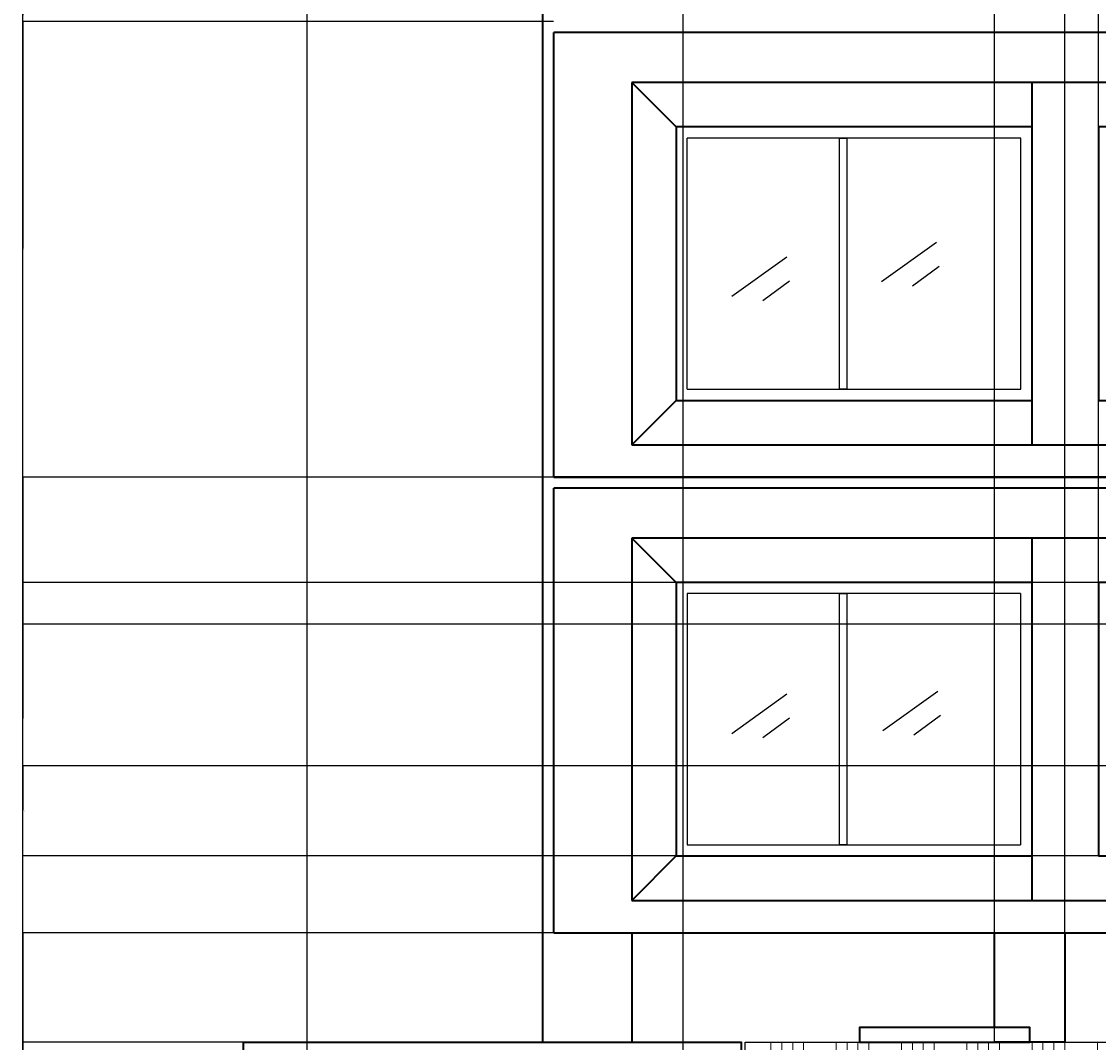
# Model space of a CAD drawing. Units: inches. Extents: x -97 to 1206, y -378 to 680.
# Tile 2 of 6: x -97 to 194, y -25 to 251. Entities that reach past the tile are written whole.
import ezdxf

# ---------------------------------------------------------------- set-up
doc = ezdxf.new("R2010")
doc.units = ezdxf.units.IN
doc.header["$MEASUREMENT"] = 0
for name, color, linetype, lineweight in [('A-ANNO-DIMS', 2, 'Continuous', 18), ('A-DOOR', 3, 'Continuous', 25), ('A-ELEV', 7, 'Continuous', 35), ('A-ELEV-PATT', 252, 'Continuous', 13), ('A-GLAZ', 4, 'Continuous', 25)]:
    doc.layers.add(name, color=color, linetype=linetype, lineweight=lineweight)
doc.styles.get("Standard").update_dxf_attribs({"font": 'arial.ttf'})
doc.dimstyles.get("Standard").update_dxf_attribs({"dimtxt": 0.18, "dimasz": 0.18, "dimexe": 0.18, "dimexo": 0.0625, "dimgap": 0.09, "dimtad": 0, "dimtih": 1, "dimtoh": 1, "dimdec": 4, "dimzin": 0, "dimdsep": 46, "dimtxsty": 'Standard', "dimcen": 0.09, "dimadec": 0, "dimazin": 0, "dimtfac": 1, "dimtdec": 4, "dimtofl": 0, "dimtmove": 0, "dimatfit": 3, "dimfxl": 1, "dimtolj": 1, "dimtzin": 0, "dimarcsym": 0})

# ---------------------------------------------------------------- blocks, each defined once
blk = doc.blocks.new('FACADE-SURROUND')
for p, q in [((432, 97.83), (0, 97.83)), ((0, 97.83), (0, 0)), ((12, 85.83), (0, 97.83)), ((300, 85.83), (312, 97.83)), ((312, 0), (312, 97.83)), ((312, 0), (312, 97.83)), ((312, 97.83), (324, 85.83)), ((432, 97.83), (420, 85.83)), ((432, 0), (432, 97.83)), ((12, 85.83), (12, 12)), ((108, 85.83), (12, 85.83)), ((300, 85.83), (126, 85.83)), ((126, 85.83), (126, 12)), ((300, 12), (300, 85.83)), ((324, 12), (324, 85.83)), ((420, 85.83), (324, 85.83)), ((420, 12), (420, 85.83)), ((12, 12), (0, 0)), ((12, 12), (108, 12)), ((126, 12), (300, 12)), ((300, 12), (312, 0)), ((312, 0), (324, 12)), ((324, 12), (420, 12)), ((432, 0), (420, 12)), ((0, 0), (432, 0))]:
    blk.add_line(p, q)
blk = doc.blocks.new('WIN-1500')
for p, q in [((90, 67.83), (0, 67.83)), ((0, 67.83), (0, 0)), ((90, 67.83), (90, 0)), ((0, 0), (90, 0))]:
    blk.add_line(p, q)
blk = doc.blocks.new('*D12')
at = {"layer": 'A-ANNO-DIMS', "color": 0, "lineweight": -2, "transparency": 16777216}
for p, q in [((43.86, 619.86), (-96.59, 619.86)), ((-96.41, 619.68), (-96.41, 252.54)), ((-96.41, -114.96), (-96.41, 252.17)), ((-36.97, -115.14), (-96.59, -115.14))]:
    blk.add_line(p, q, dxfattribs=at)
at = {"layer": 'A-ANNO-DIMS', "color": 0, "transparency": 16777216}
for points in [[(-96.44, 619.68), (-96.38, 619.68), (-96.41, 619.86)], [(-96.44, -114.96), (-96.38, -114.96), (-96.41, -115.14)]]:
    blk.add_solid(points, dxfattribs=at)
at = {"layer": 'Defpoints', "color": 0, "transparency": 16777216}
for p in [(43.93, 619.86), (-96.41, -115.14), (-36.91, -115.14)]:
    blk.add_point(p, dxfattribs=at)
at = {"layer": 'A-ANNO-DIMS', "color": 0, "transparency": 16777216, "insert": (-96.41, 252.36), "char_height": 0.18, "attachment_point": 5}
blk.add_mtext('\\A1;735', dxfattribs=at)
blk = doc.blocks.new('*D13')
at = {"layer": 'A-ANNO-DIMS', "color": 0, "lineweight": -2, "transparency": 16777216}
for p, q in [((46.86, 4.86), (-96.59, 4.86)), ((-96.41, 4.68), (-96.41, -54.96)), ((-96.41, -114.96), (-96.41, -55.33)), ((-36.97, -115.14), (-96.59, -115.14))]:
    blk.add_line(p, q, dxfattribs=at)
at = {"layer": 'A-ANNO-DIMS', "color": 0, "transparency": 16777216}
for points in [[(-96.44, 4.68), (-96.38, 4.68), (-96.41, 4.86)], [(-96.44, -114.96), (-96.38, -114.96), (-96.41, -115.14)]]:
    blk.add_solid(points, dxfattribs=at)
at = {"layer": 'Defpoints', "color": 0, "transparency": 16777216}
for p in [(46.93, 4.86), (-96.41, -115.14), (-36.91, -115.14)]:
    blk.add_point(p, dxfattribs=at)
at = {"layer": 'A-ANNO-DIMS', "color": 0, "transparency": 16777216, "insert": (-96.41, -55.14), "char_height": 0.18, "attachment_point": 5}
blk.add_mtext('\\A1;120', dxfattribs=at)
blk = doc.blocks.new('*D14')
at = {"layer": 'A-ANNO-DIMS', "color": 0, "lineweight": -2, "transparency": 16777216}
for p, q in [((46.86, 127.86), (-96.59, 127.86)), ((-96.41, 127.68), (-96.41, 66.54)), ((-96.41, 5.04), (-96.41, 66.17)), ((46.86, 4.86), (-96.59, 4.86))]:
    blk.add_line(p, q, dxfattribs=at)
at = {"layer": 'A-ANNO-DIMS', "color": 0, "transparency": 16777216}
for points in [[(-96.44, 127.68), (-96.38, 127.68), (-96.41, 127.86)], [(-96.44, 5.04), (-96.38, 5.04), (-96.41, 4.86)]]:
    blk.add_solid(points, dxfattribs=at)
at = {"layer": 'Defpoints', "color": 0, "transparency": 16777216}
for p in [(-96.41, 127.86), (46.93, 127.86), (46.93, 4.86)]:
    blk.add_point(p, dxfattribs=at)
at = {"layer": 'A-ANNO-DIMS', "color": 0, "transparency": 16777216, "insert": (-96.41, 66.36), "char_height": 0.18, "attachment_point": 5}
blk.add_mtext('\\A1;123', dxfattribs=at)
blk = doc.blocks.new('*D15')
at = {"layer": 'A-ANNO-DIMS', "color": 0, "lineweight": -2, "transparency": 16777216}
for p, q in [((46.86, 250.86), (-96.59, 250.86)), ((-96.41, 250.68), (-96.41, 189.54)), ((-96.41, 128.04), (-96.41, 189.17)), ((46.86, 127.86), (-96.59, 127.86))]:
    blk.add_line(p, q, dxfattribs=at)
at = {"layer": 'A-ANNO-DIMS', "color": 0, "transparency": 16777216}
for points in [[(-96.44, 250.68), (-96.38, 250.68), (-96.41, 250.86)], [(-96.44, 128.04), (-96.38, 128.04), (-96.41, 127.86)]]:
    blk.add_solid(points, dxfattribs=at)
at = {"layer": 'Defpoints', "color": 0, "transparency": 16777216}
for p in [(-96.41, 250.86), (46.93, 250.86), (46.93, 127.86)]:
    blk.add_point(p, dxfattribs=at)
at = {"layer": 'A-ANNO-DIMS', "color": 0, "transparency": 16777216, "insert": (-96.41, 189.36), "char_height": 0.18, "attachment_point": 5}
blk.add_mtext('\\A1;123', dxfattribs=at)
blk = doc.blocks.new('*D16')
at = {"layer": 'A-ANNO-DIMS', "color": 0, "lineweight": -2, "transparency": 16777216}
for p, q in [((46.86, 373.86), (-96.59, 373.86)), ((-96.41, 373.68), (-96.41, 312.54)), ((-96.41, 251.04), (-96.41, 312.17)), ((46.86, 250.86), (-96.59, 250.86))]:
    blk.add_line(p, q, dxfattribs=at)
at = {"layer": 'A-ANNO-DIMS', "color": 0, "transparency": 16777216}
for points in [[(-96.44, 373.68), (-96.38, 373.68), (-96.41, 373.86)], [(-96.44, 251.04), (-96.38, 251.04), (-96.41, 250.86)]]:
    blk.add_solid(points, dxfattribs=at)
at = {"layer": 'Defpoints', "color": 0, "transparency": 16777216}
for p in [(-96.41, 373.86), (46.93, 373.86), (46.93, 250.86)]:
    blk.add_point(p, dxfattribs=at)
at = {"layer": 'A-ANNO-DIMS', "color": 0, "transparency": 16777216, "insert": (-96.41, 312.36), "char_height": 0.18, "attachment_point": 5}
blk.add_mtext('\\A1;123', dxfattribs=at)
blk = doc.blocks.new('*D35')
at = {"layer": 'A-ANNO-DIMS', "color": 0, "lineweight": -2, "transparency": 16777216}
for p, q in [((-36.97, -24.73), (-96.59, -24.73)), ((-96.41, -24.91), (-96.41, -69.75)), ((-96.41, -114.96), (-96.41, -70.12)), ((-36.97, -115.14), (-96.59, -115.14))]:
    blk.add_line(p, q, dxfattribs=at)
at = {"layer": 'A-ANNO-DIMS', "color": 0, "transparency": 16777216}
for points in [[(-96.44, -24.91), (-96.38, -24.91), (-96.41, -24.73)], [(-96.44, -114.96), (-96.38, -114.96), (-96.41, -115.14)]]:
    blk.add_solid(points, dxfattribs=at)
at = {"layer": 'Defpoints', "color": 0, "transparency": 16777216}
for p in [(-96.41, -24.73), (-36.91, -24.73), (-36.91, -115.14)]:
    blk.add_point(p, dxfattribs=at)
at = {"layer": 'A-ANNO-DIMS', "color": 0, "transparency": 16777216, "insert": (-96.41, -69.94), "char_height": 0.18, "attachment_point": 5}
blk.add_mtext('\\A1;90.42', dxfattribs=at)
blk = doc.blocks.new('*D36')
at = {"layer": 'A-ANNO-DIMS', "color": 0, "lineweight": -2, "transparency": 16777216}
for p, q in [((-19.68, -48.26), (-19.68, 679.54)), ((-19.5, 679.36), (30.69, 679.36)), ((81.65, 679.36), (31.46, 679.36)), ((81.83, -48.26), (81.83, 679.54))]:
    blk.add_line(p, q, dxfattribs=at)
at = {"layer": 'A-ANNO-DIMS', "color": 0, "transparency": 16777216}
for points in [[(-19.5, 679.39), (-19.5, 679.33), (-19.68, 679.36)], [(81.65, 679.39), (81.65, 679.33), (81.83, 679.36)]]:
    blk.add_solid(points, dxfattribs=at)
at = {"layer": 'Defpoints', "color": 0, "transparency": 16777216}
for p in [(81.83, 679.36), (-19.68, -48.33), (81.83, -48.33)]:
    blk.add_point(p, dxfattribs=at)
at = {"layer": 'A-ANNO-DIMS', "color": 0, "transparency": 16777216, "insert": (31.08, 679.36), "char_height": 0.18, "attachment_point": 5}
blk.add_mtext('\\A1;101.5', dxfattribs=at)
blk = doc.blocks.new('*D40')
at = {"layer": 'A-ANNO-DIMS', "color": 0, "lineweight": -2, "transparency": 16777216}
for p, q in [((193.93, 99.46), (193.93, 679.54)), ((194.11, 679.36), (280.65, 679.36)), ((367.75, 679.36), (281.21, 679.36)), ((367.93, 99.46), (367.93, 679.54))]:
    blk.add_line(p, q, dxfattribs=at)
at = {"layer": 'A-ANNO-DIMS', "color": 0, "transparency": 16777216}
for points in [[(194.11, 679.39), (194.11, 679.33), (193.93, 679.36)], [(367.75, 679.39), (367.75, 679.33), (367.93, 679.36)]]:
    blk.add_solid(points, dxfattribs=at)
at = {"layer": 'Defpoints', "color": 0, "transparency": 16777216}
for p in [(367.93, 679.36), (193.93, 99.4), (367.93, 99.4)]:
    blk.add_point(p, dxfattribs=at)
at = {"layer": 'A-ANNO-DIMS', "color": 0, "transparency": 16777216, "insert": (280.93, 679.36), "char_height": 0.18, "attachment_point": 5}
blk.add_mtext('\\A1;174', dxfattribs=at)
blk = doc.blocks.new('*D41')
at = {"layer": 'A-ANNO-DIMS', "color": 0, "lineweight": -2, "transparency": 16777216}
for p, q in [((193.86, 99.4), (-96.59, 99.4)), ((-96.41, 99.22), (-96.41, 62.66)), ((-96.41, 25.75), (-96.41, 62.3)), ((193.86, 25.57), (-96.59, 25.57))]:
    blk.add_line(p, q, dxfattribs=at)
at = {"layer": 'A-ANNO-DIMS', "color": 0, "transparency": 16777216}
for points in [[(-96.44, 99.22), (-96.38, 99.22), (-96.41, 99.4)], [(-96.44, 25.75), (-96.38, 25.75), (-96.41, 25.57)]]:
    blk.add_solid(points, dxfattribs=at)
at = {"layer": 'Defpoints', "color": 0, "transparency": 16777216}
for p in [(-96.41, 99.4), (193.93, 99.4), (193.93, 25.57)]:
    blk.add_point(p, dxfattribs=at)
at = {"layer": 'A-ANNO-DIMS', "color": 0, "transparency": 16777216, "insert": (-96.41, 62.48), "char_height": 0.18, "attachment_point": 5}
blk.add_mtext('\\A1;73.83', dxfattribs=at)
blk = doc.blocks.new('*D42')
at = {"layer": 'A-ANNO-DIMS', "color": 0, "lineweight": -2, "transparency": 16777216}
for p, q in [((193.86, 49.88), (-96.59, 49.88)), ((-96.41, 49.7), (-96.41, 37.91)), ((-96.41, 25.75), (-96.41, 37.54)), ((193.86, 25.57), (-96.59, 25.57))]:
    blk.add_line(p, q, dxfattribs=at)
at = {"layer": 'A-ANNO-DIMS', "color": 0, "transparency": 16777216}
for points in [[(-96.44, 49.7), (-96.38, 49.7), (-96.41, 49.88)], [(-96.44, 25.75), (-96.38, 25.75), (-96.41, 25.57)]]:
    blk.add_solid(points, dxfattribs=at)
at = {"layer": 'Defpoints', "color": 0, "transparency": 16777216}
for p in [(-96.41, 49.88), (193.93, 49.88), (193.93, 25.57)]:
    blk.add_point(p, dxfattribs=at)
at = {"layer": 'A-ANNO-DIMS', "color": 0, "transparency": 16777216, "insert": (-96.41, 37.72), "char_height": 0.18, "attachment_point": 5}
blk.add_mtext('\\A1;24.314', dxfattribs=at)
blk = doc.blocks.new('*D44')
at = {"layer": 'A-ANNO-DIMS', "color": 0, "lineweight": -2, "transparency": 16777216}
for p, q in [((262.43, 88.15), (-96.59, 88.15)), ((-96.41, 87.97), (-96.41, 69.2)), ((-96.41, 50.06), (-96.41, 68.83)), ((262.43, 49.88), (-96.59, 49.88))]:
    blk.add_line(p, q, dxfattribs=at)
at = {"layer": 'A-ANNO-DIMS', "color": 0, "transparency": 16777216}
for points in [[(-96.44, 87.97), (-96.38, 87.97), (-96.41, 88.15)], [(-96.44, 50.06), (-96.38, 50.06), (-96.41, 49.88)]]:
    blk.add_solid(points, dxfattribs=at)
at = {"layer": 'Defpoints', "color": 0, "transparency": 16777216}
for p in [(-96.41, 88.15), (262.49, 88.15), (262.49, 49.88)]:
    blk.add_point(p, dxfattribs=at)
at = {"layer": 'A-ANNO-DIMS', "color": 0, "transparency": 16777216, "insert": (-96.41, 69.01), "char_height": 0.18, "attachment_point": 5}
blk.add_mtext('\\A1;38.266', dxfattribs=at)
blk = doc.blocks.new('*D45')
at = {"layer": 'A-ANNO-DIMS', "color": 0, "lineweight": -2, "transparency": 16777216}
for p, q in [((43.93, -24.66), (43.93, 679.54)), ((44.11, 679.36), (104.5, 679.36)), ((165.65, 679.36), (105.27, 679.36)), ((165.83, -24.66), (165.83, 679.54))]:
    blk.add_line(p, q, dxfattribs=at)
at = {"layer": 'A-ANNO-DIMS', "color": 0, "transparency": 16777216}
for points in [[(44.11, 679.39), (44.11, 679.33), (43.93, 679.36)], [(165.65, 679.39), (165.65, 679.33), (165.83, 679.36)]]:
    blk.add_solid(points, dxfattribs=at)
at = {"layer": 'Defpoints', "color": 0, "transparency": 16777216}
for p in [(165.83, 679.36), (43.93, -24.73), (165.83, -24.73)]:
    blk.add_point(p, dxfattribs=at)
at = {"layer": 'A-ANNO-DIMS', "color": 0, "transparency": 16777216, "insert": (104.88, 679.36), "char_height": 0.18, "attachment_point": 5}
blk.add_mtext('\\A1;121.9', dxfattribs=at)
blk = doc.blocks.new('*D46')
at = {"layer": 'A-ANNO-DIMS', "color": 0, "lineweight": -2, "transparency": 16777216}
for p, q in [((165.83, -24.66), (165.83, 679.54)), ((166.01, 679.36), (174.88, 679.36)), ((184.65, 679.36), (175.79, 679.36)), ((184.83, -24.66), (184.83, 679.54))]:
    blk.add_line(p, q, dxfattribs=at)
at = {"layer": 'A-ANNO-DIMS', "color": 0, "transparency": 16777216}
for points in [[(166.01, 679.39), (166.01, 679.33), (165.83, 679.36)], [(184.65, 679.39), (184.65, 679.33), (184.83, 679.36)]]:
    blk.add_solid(points, dxfattribs=at)
at = {"layer": 'Defpoints', "color": 0, "transparency": 16777216}
for p in [(184.83, 679.36), (165.83, -24.73), (184.83, -24.73)]:
    blk.add_point(p, dxfattribs=at)
at = {"layer": 'A-ANNO-DIMS', "color": 0, "transparency": 16777216, "insert": (175.33, 679.36), "char_height": 0.18, "attachment_point": 5}
blk.add_mtext('\\A1;18.994', dxfattribs=at)
blk = doc.blocks.new('*D47')
at = {"layer": 'A-ANNO-DIMS', "color": 0, "lineweight": -2, "transparency": 16777216}
for p, q in [((184.83, -24.66), (184.83, 679.54)), ((185.01, 679.36), (255.01, 679.36)), ((325.75, 679.36), (255.75, 679.36)), ((325.93, -24.66), (325.93, 679.54))]:
    blk.add_line(p, q, dxfattribs=at)
at = {"layer": 'A-ANNO-DIMS', "color": 0, "transparency": 16777216}
for points in [[(185.01, 679.39), (185.01, 679.33), (184.83, 679.36)], [(325.75, 679.39), (325.75, 679.33), (325.93, 679.36)]]:
    blk.add_solid(points, dxfattribs=at)
at = {"layer": 'Defpoints', "color": 0, "transparency": 16777216}
for p in [(325.93, 679.36), (184.83, -24.73), (325.93, -24.73)]:
    blk.add_point(p, dxfattribs=at)
at = {"layer": 'A-ANNO-DIMS', "color": 0, "transparency": 16777216, "insert": (255.38, 679.36), "char_height": 0.18, "attachment_point": 5}
blk.add_mtext('\\A1;141.1', dxfattribs=at)

msp = doc.modelspace()

# ---------------------------------------------------------------- hatches: boundary and pattern name
at = {"layer": 'A-ELEV-PATT'}
h = msp.add_hatch(dxfattribs=at)
h.set_pattern_fill('HOUND', color=256, scale=47)
h.set_pattern_definition([(0, (-208.809, -191.922), (11.75, 2.9375), [47, -23.5]), (90, (-208.809, -191.922), (-2.9375, -11.75), [47, -23.5])])
h.paths.add_polyline_path([(81.8295, -48.3264), (-19.6789, -48.3264), (-19.6789, -97.3647), (81.8295, -97.3647)])
h.paths.add_polyline_path([(-8.2183, -60.8667), (63.8199, -60.8667), (63.8199, -84.3116), (-8.2183, -84.3116)], flags=16)
h.paths.add_polyline_path([(403.1688, -24.8426), (391.3618, -24.8426), (391.3618, -84.5669), (507.9182, -84.5669), (507.9182, -24.8426), (495.2029, -24.8426), (495.2029, -75.7956), (403.1688, -75.7956)])
h.paths.add_polyline_path([(430.113, -24.8426), (421.6362, -24.8426), (421.6362, -57.6481), (478.552, -57.6481), (478.552, -24.8426), (469.7725, -24.8426), (469.7725, -49.4817), (430.113, -49.4817)], flags=17)
h.paths.add_polyline_path([(378.6527, -24.7259), (98.5594, -24.7259), (98.5594, -27.0887), (378.6527, -27.0887)])
h.paths.add_polyline_path([(177.3114, -53.6191), (173.9058, -53.6191), (173.9058, -63.7423), (177.3114, -63.7423)])
h.paths.add_polyline_path([(177.3114, -63.7423), (173.9058, -63.7423), (173.9058, -69.9353), (177.3114, -69.9353)])
h.paths.add_polyline_path([(290.4371, -69.9353), (286.815, -69.9353), (286.815, -74.3824), (290.4371, -74.3824)])
h.paths.add_polyline_path([(290.4371, -63.7423), (286.815, -63.7423), (286.815, -69.9353), (290.4371, -69.9353)])
h.paths.add_polyline_path([(290.4371, -53.6191), (286.815, -53.6191), (286.815, -63.7423), (290.4371, -63.7423)])
h.paths.add_polyline_path([(290.4371, -50.7545), (286.815, -50.7545), (286.815, -53.6191), (290.4371, -53.6191)])

# ---------------------------------------------------------------- linework, layer by layer
at = {"layer": 'A-DOOR'}
msp.add_lwpolyline([(98.5594, -24.7259), (378.6527, -24.7259), (378.6527, -115.1448), (98.5594, -115.1448)], close=True, dxfattribs=at)
at = {"layer": 'A-ELEV'}
for p, q in [((43.9261, 4.8552), (43.9261, 619.8552)), ((523.9261, 247.8552), (46.9261, 247.8552)), ((46.9261, 127.8552), (46.9261, 247.8552)), ((175.9261, 234.3966), (175.9261, 136.5671)), ((523.9261, 127.8552), (46.9261, 127.8552)), ((46.9261, 127.8552), (523.9261, 127.8552)), ((523.9261, 124.8552), (46.9261, 124.8552)), ((46.9261, 4.8552), (46.9261, 124.8552)), ((175.9261, 111.3966), (175.9261, 13.5671)), ((46.9261, 4.8552), (523.9261, 4.8552)), ((67.9261, 4.8552), (67.9261, -24.7259))]:
    msp.add_line(p, q, dxfattribs=at)
for points in [[(46.9261, 4.8552), (524.19, 4.8552), (524.19, -115.1448), (43.9261, -115.1448)], [(43.9261, -24.7259), (43.9261, 4.8552)], [(165.835, -20.7683), (165.835, 4.8552), (184.8288, 4.8552), (184.8288, -24.7259), (165.835, -24.7259)]]:
    msp.add_lwpolyline(points, dxfattribs=at)
for points in [[(129.4209, -24.7259), (175.3958, -24.7259), (175.3958, -20.7683), (129.4209, -20.7683)], [(-36.9051, -24.7259), (97.4484, -24.7259), (97.4484, -115.1448), (-36.9051, -115.1448)]]:
    msp.add_lwpolyline(points, close=True, dxfattribs=at)
at = {"layer": 'A-GLAZ'}
for p, q in [((135.3178, 180.6447), (150.1751, 191.3014)), ((94.9363, 176.6989), (109.7936, 187.3556)), ((143.6988, 179.5029), (150.937, 184.8313)), ((103.3174, 175.5571), (110.5556, 180.8855)), ((135.6956, 59.4248), (150.5529, 70.0816)), ((94.9332, 58.6636), (109.7905, 69.3204)), ((103.3143, 57.5219), (110.5524, 62.8502)), ((144.0767, 58.2831), (151.3148, 63.6114))]:
    msp.add_line(p, q, dxfattribs=at)
for points in [[(124.0501, 219.3966), (126.0187, 219.3966), (126.0187, 151.5671), (124.0501, 151.5671)], [(124.0501, 96.3966), (126.0187, 96.3966), (126.0187, 28.5671), (124.0501, 28.5671)]]:
    msp.add_lwpolyline(points, close=True, dxfattribs=at)

# ---------------------------------------------------------------- block references
at = {"layer": 'A-ELEV'}
for p in [(67.926, 136.567), (67.926, 13.567)]:
    msp.add_blockref('FACADE-SURROUND', p, dxfattribs=at)
at = {"layer": 'A-GLAZ', "rotation": 180}
msp.add_blockref('WIN-1500', (172.9262, 219.3967), dxfattribs=at)
at = {"layer": 'A-GLAZ'}
msp.add_blockref('WIN-1500', (82.926, 28.567), dxfattribs=at)

# ---------------------------------------------------------------- dimensions: what is measured, and where the dimension line sits
at = {"layer": 'A-ANNO-DIMS'}
for base, p1, p2, override, picture, middle in [((81.8295, 679.3552), (-19.6789, -48.3264), (81.8295, -48.3264), {"dimdec": 1, "dimlfac": 1, "dimrnd": 0, "dimzin": 0, "dimdsep": 46, "dimlunit": 2}, '*D36', (31.0753, 679.3552)), ((165.835, 679.3552), (43.9261, -24.7259), (165.835, -24.7259), {"dimdec": 1, "dimlfac": 1, "dimrnd": 0, "dimzin": 0, "dimdsep": 46, "dimlunit": 2}, '*D45', (104.8805, 679.3552)), ((184.8288, 679.3552), (165.835, -24.7259), (184.8288, -24.7259), {"dimdec": 3, "dimlfac": 1, "dimrnd": 0, "dimzin": 0, "dimdsep": 46, "dimlunit": 2}, '*D46', (175.3319, 679.3552)), ((325.9258, 679.3552), (184.8288, -24.7259), (325.9258, -24.7259), {"dimdec": 1, "dimlfac": 1, "dimrnd": 0, "dimzin": 0, "dimdsep": 46, "dimlunit": 2}, '*D47', (255.3773, 679.3552)), ((367.9261, 679.3552), (193.9261, 99.3966), (367.9261, 99.3966), {"dimdec": 0, "dimlfac": 1, "dimrnd": 0, "dimzin": 0, "dimdsep": 46, "dimlunit": 2}, '*D40', (280.9261, 679.3552))]:
    dim = msp.add_linear_dim(base=base, p1=p1, p2=p2, dimstyle='Standard', override=override, dxfattribs=at)
    dim.commit()
    dim.dimension.update_dxf_attribs({"geometry": picture, "text_midpoint": middle})
for base, p1, p2, override, picture, middle in [((-96.4051, -115.1448), (43.9261, 619.8552), (-36.9051, -115.1448), {"dimdec": 0, "dimlfac": 1, "dimrnd": 0, "dimzin": 0, "dimdsep": 46, "dimlunit": 2}, '*D12', (-96.4051, 252.3552)), ((-96.4051, 373.8552), (46.9261, 250.8552), (46.9261, 373.8552), {"dimdec": 0, "dimlfac": 1, "dimrnd": 0, "dimzin": 0, "dimdsep": 46, "dimlunit": 2}, '*D16', (-96.4051, 312.3552)), ((-96.4051, 250.8552), (46.9261, 127.8552), (46.9261, 250.8552), {"dimdec": 0, "dimlfac": 1, "dimrnd": 0, "dimzin": 0, "dimdsep": 46, "dimlunit": 2}, '*D15', (-96.4051, 189.3552)), ((-96.4051, 127.8552), (46.9261, 4.8552), (46.9261, 127.8552), {"dimdec": 0, "dimlfac": 1, "dimrnd": 0, "dimzin": 0, "dimdsep": 46, "dimlunit": 2}, '*D14', (-96.4051, 66.3552)), ((-96.4051, 99.3966), (193.9261, 25.5671), (193.9261, 99.3966), {"dimdec": 2, "dimlfac": 1, "dimrnd": 0, "dimzin": 0, "dimdsep": 46, "dimlunit": 2}, '*D41', (-96.4051, 62.4819)), ((-96.4051, 88.1471), (262.4936, 49.8815), (262.4936, 88.1471), {"dimdec": 3, "dimlfac": 1, "dimrnd": 0, "dimzin": 0, "dimdsep": 46, "dimlunit": 2}, '*D44', (-96.4051, 69.0143)), ((-96.4051, 49.8815), (193.9261, 25.5671), (193.9261, 49.8815), {"dimdec": 3, "dimlfac": 1, "dimrnd": 0, "dimzin": 0, "dimdsep": 46, "dimlunit": 2}, '*D42', (-96.4051, 37.7243)), ((-96.4051, -115.1448), (46.9261, 4.8552), (-36.9051, -115.1448), {"dimdec": 0, "dimlfac": 1, "dimrnd": 0, "dimzin": 0, "dimdsep": 46, "dimlunit": 2}, '*D13', (-96.4051, -55.1448)), ((-96.4051, -24.7259), (-36.9051, -115.1448), (-36.9051, -24.7259), {"dimdec": 2, "dimlfac": 1, "dimrnd": 0, "dimzin": 0, "dimdsep": 46, "dimlunit": 2}, '*D35', (-96.4051, -69.9353))]:
    dim = msp.add_linear_dim(base=base, p1=p1, p2=p2, angle=90, dimstyle='Standard', override=override, dxfattribs=at)
    dim.commit()
    dim.dimension.update_dxf_attribs({"geometry": picture, "text_midpoint": middle})

doc.saveas('drawing.dxf')
